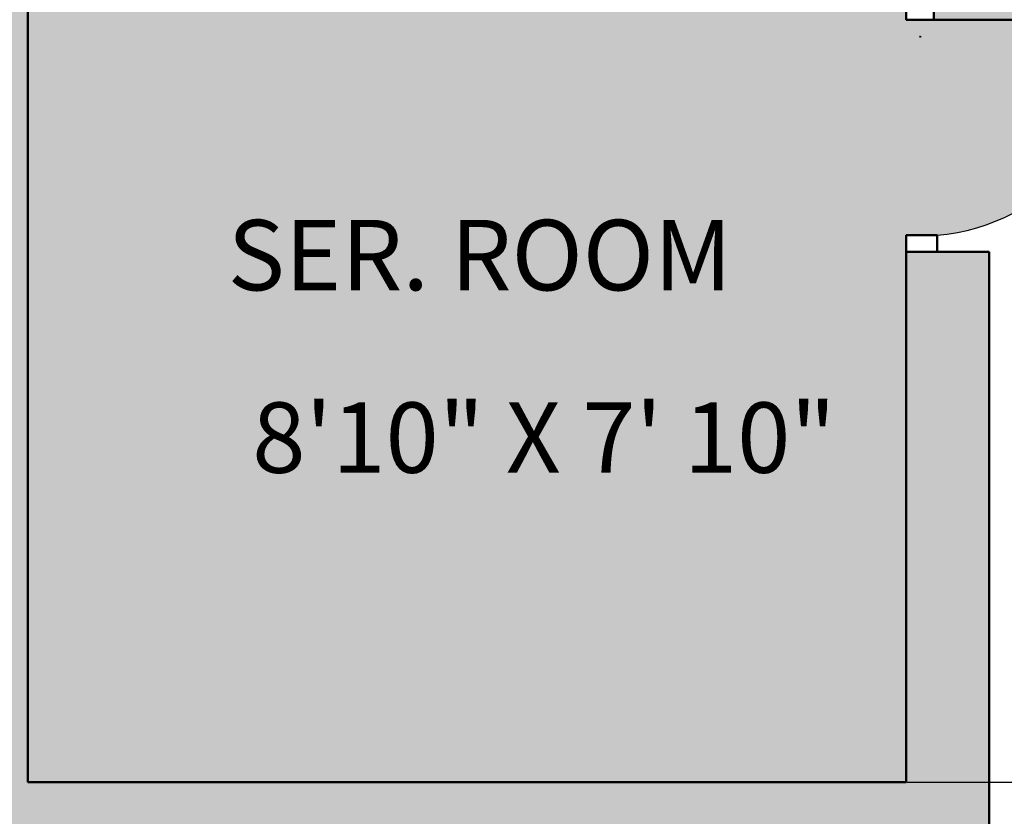
# Model space of a CAD drawing. Units: inches. Extents: x 925 to 2834, y 111 to 1355.
# Tile 9 of 25: x 1602 to 1721, y 723 to 820. Entities that reach past the tile are written whole.
import ezdxf

# ---------------------------------------------------------------- set-up
doc = ezdxf.new("R2010")
doc.units = ezdxf.units.IN
doc.header["$MEASUREMENT"] = 0
for name, color, linetype, lineweight in [('A-ANNO-DIMS', 2, 'Continuous', 18), ('A-AREA-IDEN', 7, 'Continuous', 18), ('A-DOOR', 2, 'Continuous', 25), ('A-FLOR-PATT', 252, 'Continuous', 13), ('A-WALL', 7, 'Continuous', 50)]:
    doc.layers.add(name, color=color, linetype=linetype, lineweight=lineweight)
doc.styles.get("Standard").update_dxf_attribs({"font": 'arial.ttf'})
doc.dimstyles.get("Standard").update_dxf_attribs({"dimtxt": 6, "dimasz": 3, "dimexe": 0.18, "dimexo": 0.0625, "dimgap": 0.09, "dimtad": 0, "dimtih": 1, "dimtoh": 1, "dimdec": 1, "dimzin": 0, "dimdsep": 46, "dimlunit": 3, "dimtxsty": 'Standard', "dimblk": 'ARCHTICK', "dimcen": 0.09, "dimadec": 0, "dimazin": 0, "dimtfac": 1, "dimtdec": 1, "dimtofl": 0, "dimtmove": 0, "dimatfit": 3, "dimfxl": 1, "dimtolj": 1, "dimtzin": 0, "dimarcsym": 0})

# ---------------------------------------------------------------- blocks, each defined once
blk = doc.blocks.new('_ArchTick')
at = {"color": 0, "linetype": 'ByBlock', "const_width": 0.15}
blk.add_lwpolyline([(-0.5, -0.5), (0.5, 0.5)], dxfattribs=at)
blk = doc.blocks.new('*D45')
at = {"layer": 'A-ANNO-DIMS', "color": 0, "lineweight": -2, "transparency": 16777216}
for p, q in [((1708.78, 727.59), (1988.62, 727.59)), ((1988.44, 727.59), (1988.44, 687.74)), ((1988.44, 641.59), (1988.44, 681.44)), ((1708.78, 641.59), (1988.62, 641.59))]:
    blk.add_line(p, q, dxfattribs=at)
at = {"layer": 'Defpoints', "color": 0, "transparency": 16777216}
for p in [(1708.71, 727.59), (1988.44, 727.59), (1708.71, 641.59)]:
    blk.add_point(p, dxfattribs=at)
at = {"layer": 'A-ANNO-DIMS', "color": 0, "lineweight": -2, "transparency": 16777216, "xscale": 3, "yscale": 3, "zscale": 3}
for p, rotation in [((1988.44, 727.59), 90), ((1988.44, 641.59), 270)]:
    blk.add_blockref('_ArchTick', p, dxfattribs=dict(at, rotation=rotation))
at = {"layer": 'A-ANNO-DIMS', "color": 0, "transparency": 16777216, "insert": (1988.44, 684.59), "char_height": 6, "attachment_point": 5}
blk.add_mtext('\\A1;86', dxfattribs=at)
blk = doc.blocks.new('*D46')
at = {"layer": 'A-ANNO-DIMS', "color": 0, "lineweight": -2, "transparency": 16777216}
for p, q in [((1708.78, 828.59), (1988.62, 828.59)), ((1988.44, 828.59), (1988.44, 781.24)), ((1988.44, 727.59), (1988.44, 774.94)), ((1708.78, 727.59), (1988.62, 727.59))]:
    blk.add_line(p, q, dxfattribs=at)
at = {"layer": 'Defpoints', "color": 0, "transparency": 16777216}
for p in [(1708.71, 828.59), (1988.44, 828.59), (1708.71, 727.59)]:
    blk.add_point(p, dxfattribs=at)
at = {"layer": 'A-ANNO-DIMS', "color": 0, "lineweight": -2, "transparency": 16777216, "xscale": 3, "yscale": 3, "zscale": 3}
for p, rotation in [((1988.44, 828.59), 90), ((1988.44, 727.59), 270)]:
    blk.add_blockref('_ArchTick', p, dxfattribs=dict(at, rotation=rotation))
at = {"layer": 'A-ANNO-DIMS', "color": 0, "transparency": 16777216, "insert": (1988.44, 778.09), "char_height": 6, "attachment_point": 5}
blk.add_mtext('\\A1;101', dxfattribs=at)
blk = doc.blocks.new('*D82')
at = {"layer": 'A-ANNO-DIMS', "color": 0, "lineweight": -2, "transparency": 16777216}
for p, q in [((1710.41, 817.46), (1710.41, 817.64)), ((1710.32, 817.55), (1710.5, 817.55)), ((1739.82, 792.74), (1728.79, 802.05)), ((1742.82, 792.74), (1739.82, 792.74))]:
    blk.add_line(p, q, dxfattribs=at)
at = {"layer": 'Defpoints', "color": 0, "transparency": 16777216}
for p in [(1710.41, 817.55), (1728.79, 802.05)]:
    blk.add_point(p, dxfattribs=at)
at = {"layer": 'A-ANNO-DIMS', "color": 0, "lineweight": -2, "transparency": 16777216, "xscale": 3, "yscale": 3, "zscale": 3, "rotation": 139.8500923460391}
blk.add_blockref('_ArchTick', (1728.79, 802.05), dxfattribs=at)
at = {"layer": 'A-ANNO-DIMS', "color": 0, "transparency": 16777216, "insert": (1762.43, 792.74), "char_height": 6, "attachment_point": 5}
blk.add_mtext('\\A1;2X R24.05', dxfattribs=at)

msp = doc.modelspace()

# ---------------------------------------------------------------- hatches: boundary and pattern name
at = {"layer": 'A-FLOR-PATT', "transparency": 33554605}
h = msp.add_hatch(color=256, dxfattribs=at)
h.dxf.hatch_style = 1
h.paths.add_polyline_path([(1931.688, 1294.5638), (991.7375, 1294.5638), (991.7375, 172.1134), (1931.688, 172.1134)])
h.paths.add_polyline_path([(1910.7128, 1273.5886), (1910.7128, 193.0886), (1012.7128, 193.0886), (1012.7128, 1273.5886)], flags=16)
h.paths.add_polyline_path([(1850.7128, 1213.5886), (1850.7128, 253.0886), (1072.7128, 253.0886), (1072.7128, 1213.5886)], flags=0)
h.paths.add_polyline_path([(1838.7128, 1201.5886), (1838.7128, 265.0886), (1084.7128, 265.0886), (1084.7128, 530.5886), (1084.7128, 1201.5886)], flags=0)
h.paths.add_polyline_path([(1547.6758, 1155.7396), (1547.6758, 1119.115), (1513.0687, 1119.115), (1513.0687, 1155.7396)], flags=0)
h.paths.add_polyline_path([(1600.1067, 1154.9439), (1634.7139, 1154.9439), (1634.7139, 1119.115), (1600.1067, 1119.115)], flags=0)
h.paths.add_polyline_path([(1505.2502, 1144.5358), (1505.2502, 1119.115), (1470.643, 1119.115), (1470.643, 1144.5358)], flags=0)
h.paths.add_polyline_path([(1559.1357, 1141.0962), (1593.7428, 1141.0962), (1593.7428, 1119.115), (1559.1357, 1119.115)], flags=0)
h.paths.add_polyline_path([(1462.8966, 1154.9439), (1462.8966, 1119.115), (1428.2895, 1119.115), (1428.2895, 1154.9439)], flags=0)
h.paths.add_polyline_path([(1642.4603, 1144.5358), (1677.0675, 1144.5358), (1677.0675, 1119.115), (1642.4603, 1119.115)], flags=0)
h.paths.add_polyline_path([(1422.3508, 1141.0962), (1422.3508, 1119.115), (1387.7436, 1119.115), (1387.7436, 1141.0962)], flags=0)
h.paths.add_polyline_path([(1684.8859, 1155.7396), (1719.4931, 1155.7396), (1719.4931, 1119.115), (1684.8859, 1119.115)], flags=0)
h.paths.add_polyline_path([(1718.7128, 1081.5886), (1718.7128, 1050.1249), (1715.7128, 1050.1249), (1715.7128, 1026.1249), (1715.7128, 1002.1249), (1718.7128, 1002.1249), (1730.7128, 1002.1249), (1730.7128, 998.1249), (1730.7128, 990.1249), (1730.7128, 986.1249), (1718.7128, 986.1249), (1718.7128, 893.5886), (1715.3735, 893.5886), (1715.3735, 891.5886), (1713.3735, 891.5886, 0.41421356), (1677.3735, 855.5886), (1713.3735, 855.5886), (1713.3735, 853.5886), (1715.3735, 853.5886), (1715.3735, 851.5886), (1718.7128, 851.5886), (1718.7128, 821.5865), (1734.4655, 821.5865), (1734.3735, 819.5886, -0.41421356), (1712.4415, 793.5886), (1712.4415, 791.5886), (1718.7128, 791.5886), (1718.7128, 717.5886), (1718.7128, 669.5886), (1732.7128, 669.5886), (1732.7128, 665.5886), (1732.7128, 641.5886), (1732.7128, 634.5886), (1732.7128, 610.5886), (1732.7128, 603.5886), (1718.7128, 603.5886), (1718.7128, 385.0886), (1434.2128, 385.0886), (1434.2128, 530.5886), (1410.2128, 530.5886), (1408.2128, 530.5886), (1408.2128, 532.5886, 0.41421356), (1372.2128, 568.5886), (1372.2128, 532.5886), (1370.2128, 532.5886), (1370.2128, 530.5886), (1368.2128, 530.5886), (1282.2128, 530.5886), (1210.2128, 530.5886), (1200.2128, 530.5886), (1200.2128, 542.1915), (1183.2307, 542.1915), (1183.2307, 546.1915), (1200.2128, 546.1915), (1200.2128, 572.1915), (1183.2307, 572.1915), (1183.2307, 576.1915), (1200.2128, 576.1915), (1200.2128, 727.5886), (1210.2128, 727.5886), (1234.2128, 727.5886), (1259.7128, 727.5886), (1259.7128, 775.5886), (1259.7128, 799.5886), (1259.7128, 847.5886), (1259.7128, 993.5872), (1259.7128, 1065.5872), (1259.7128, 1071.5886), (1219.6318, 1071.5886), (1219.6318, 1081.5886), (1084.7128, 1081.5886), (1084.7128, 1119.115), (1256.8974, 1119.115), (1256.8974, 1154.9439), (1291.5046, 1154.9439), (1291.5046, 1119.115), (1256.8974, 1119.115), (1256.6723, 1081.5886), (1293.7128, 1081.5886), (1341.7128, 1081.5886), (1341.7128, 1093.5886), (1347.7128, 1093.5886), (1371.7128, 1093.5886), (1377.7128, 1093.5886), (1377.7128, 1081.5886), (1668.7128, 1081.5886), (1668.7128, 1117.5886), (1675.7128, 1117.5886), (1711.7128, 1117.5886), (1718.7128, 1117.5886)], flags=0)
h.paths.add_polyline_path([(1376.2838, 1155.7396), (1376.2838, 1119.115), (1341.6766, 1119.115), (1341.6766, 1155.7396)], flags=0)
h.paths.add_polyline_path([(1341.7128, 1076.0886), (1293.7128, 1076.0886), (1293.7128, 1071.5886), (1269.7128, 1071.5886), (1269.7128, 1065.5872), (1266.7128, 1065.5872), (1266.7128, 1029.5872), (1265.7128, 1029.5872), (1265.7128, 993.5872), (1269.7128, 993.5872), (1269.7128, 903.5886), (1269.7128, 893.5886), (1269.7128, 847.5886), (1265.2128, 847.5886), (1265.2128, 799.5886), (1269.7128, 799.5886), (1269.7128, 775.5886), (1265.2128, 775.5886), (1265.2128, 727.5886), (1269.7128, 727.5886), (1444.2128, 727.5886), (1444.2128, 717.5886), (1234.2128, 717.5886), (1234.2128, 722.0886), (1210.2128, 722.0886), (1210.2128, 717.5886), (1210.2128, 540.5886), (1210.2128, 536.0886), (1282.2128, 536.0886), (1282.2128, 535.0886), (1210.2128, 535.0886), (1210.2128, 540.5886), (1210.2128, 717.5886), (1210.2128, 723.0886), (1234.2128, 723.0886), (1234.2128, 717.5886), (1444.2128, 717.5886), (1444.2128, 727.5886), (1269.7128, 727.5886), (1264.2128, 727.5886), (1264.2128, 775.5886), (1269.7128, 775.5886), (1269.7128, 799.5886), (1264.2128, 799.5886), (1264.2128, 847.5886), (1269.7128, 847.5886), (1269.7128, 893.5886), (1269.7128, 903.5886), (1269.7128, 993.5872), (1264.7128, 993.5872), (1264.7128, 1029.5872), (1265.7128, 1029.5872), (1265.7128, 1065.5872), (1269.7128, 1065.5872), (1269.7128, 1071.5886), (1293.7128, 1071.5886), (1293.7128, 1077.0886), (1341.7128, 1077.0886)], flags=0)
h.paths.add_polyline_path([(1730.9529, 1141.0962), (1765.5601, 1141.0962), (1765.5601, 1119.115), (1730.9529, 1119.115)], flags=0)
h.paths.add_polyline_path([(1333.8582, 1144.5358), (1333.8582, 1119.115), (1299.251, 1119.115), (1299.251, 1144.5358)], flags=0)
h.paths.add_polyline_path([(1592.7128, 968.5886), (1596.0342, 968.5886), (1602.7128, 968.5886), (1708.7128, 968.5886), (1708.7128, 903.5886), (1602.7128, 903.5886), (1602.7128, 938.5886), (1592.7128, 938.5886), (1592.7128, 903.5886), (1451.7128, 903.5886), (1451.7128, 893.5886), (1511.7128, 893.5886), (1511.7128, 881.5886), (1515.2128, 881.5886), (1518.7128, 881.5886), (1518.7128, 893.5886), (1592.7128, 893.5886), (1592.7128, 799.5886), (1518.7128, 799.5886), (1518.7128, 857.5886), (1511.7128, 857.5886), (1511.7128, 799.5886), (1511.7128, 772.0886), (1521.7128, 772.0886), (1521.7128, 792.5886), (1592.7128, 792.5886), (1592.7128, 727.5886), (1521.7128, 727.5886), (1521.7128, 748.0886), (1511.7128, 748.0886), (1511.7128, 717.5886), (1708.7128, 717.5886), (1714.2128, 717.5886), (1714.2128, 669.5886), (1708.7128, 669.5886), (1708.7128, 641.5886), (1492.2128, 641.5886), (1492.2128, 631.5886), (1621.2128, 631.5886), (1621.2128, 443.0886), (1625.7128, 443.0886), (1625.7128, 503.0886), (1625.7128, 507.5886), (1625.7128, 631.5886), (1708.7128, 631.5886), (1708.7128, 507.5886), (1655.7128, 507.5886), (1655.7128, 503.0886), (1708.7128, 503.0886), (1708.7128, 395.0886), (1625.7128, 395.0886), (1625.7128, 419.0886), (1621.2128, 419.0886), (1621.2128, 395.0886), (1482.2128, 395.0886), (1482.2128, 385.0886), (1434.2128, 385.0886), (1434.2128, 433.0886), (1444.2128, 433.0886), (1444.2128, 631.5886), (1450.2128, 631.5886), (1450.2128, 634.91), (1452.2128, 634.91), (1452.2128, 669.5886), (1454.2128, 669.5886, -0.40021217), (1490.1712, 635.3173), (1492.2128, 635.3173), (1492.2128, 641.5886), (1564.7128, 641.5886), (1564.7128, 677.5886), (1672.7128, 677.5886), (1672.7128, 681.5886), (1564.7128, 681.5886), (1564.7128, 717.5886), (1511.7128, 717.5886), (1511.7128, 748.0886), (1511.7128, 772.0886), (1511.7128, 799.5886), (1511.7128, 857.5886), (1511.8913, 857.5886), (1511.8913, 859.5886), (1515.6201, 859.5886, 0.41421356), (1537.552, 879.5886), (1513.552, 879.5886), (1511.8913, 879.5886), (1511.8913, 881.5886), (1511.7128, 881.5886), (1511.7128, 893.5886), (1451.7128, 893.5886), (1451.7128, 903.5886), (1592.7128, 903.5886), (1592.7128, 938.5886), (1592.7128, 940.5886), (1596.4415, 940.5886, 0.41421356), (1618.3735, 966.5886), (1594.3735, 966.5886), (1592.7128, 966.5886)], flags=0)
h.paths.add_polyline_path([(1377.7128, 903.5886), (1377.7128, 893.5886), (1305.7128, 893.5886), (1305.7128, 903.5886)], flags=0)
h.paths.add_polyline_path([(1708.7128, 821.5886), (1712.0342, 821.5886), (1712.0342, 819.5886), (1710.3735, 819.5886), (1708.7128, 819.5886)], flags=0)
h.paths.add_polyline_path([(1576.7128, 695.1992), (1575.5896, 693.6649), (1575.9687, 694.6994), (1575.4438, 695.1992), (1575.9687, 695.699), (1575.5896, 696.7335)], flags=0)
h.paths.add_polyline_path([(1565.9817, 662.3134), (1565.4568, 661.8136), (1565.8359, 660.7791), (1564.7128, 662.3134), (1565.8359, 663.8477), (1565.4568, 662.8132)], flags=0)
h.paths.add_polyline_path([(1444.2128, 433.0886), (1444.2128, 395.0886), (1482.2128, 395.0886), (1482.2128, 389.0886), (1438.2128, 389.0886), (1438.2128, 391.8608), (1438.2128, 433.0886)], flags=0)
h.paths.add_polyline_path([(1410.2128, 506.5886), (1410.2128, 289.0886), (1108.7128, 289.0886), (1108.7128, 506.5886)], flags=0)
h.paths.add_polyline_path([(1612.3153, 838.3016), (1680.4151, 838.3016), (1680.4151, 851.3131), (1612.3153, 851.3131)], flags=8)
h.paths.add_polyline_path([(1208.3174, 395.0436), (1282.1017, 395.0436), (1282.1017, 408.0552), (1208.3174, 408.0552)], flags=8)
h.paths.add_polyline_path([(1291.8049, 598.7427), (1369.8017, 598.7427), (1369.8017, 611.7542), (1291.8049, 611.7542)], flags=8)
h.paths.add_polyline_path([(1119.679, 917.3022), (1191.0817, 917.3022), (1191.0817, 930.3137), (1119.679, 930.3137)], flags=8)
h.paths.add_polyline_path([(1332.2261, 815.9808), (1410.2258, 815.9808), (1410.2258, 829.001), (1332.2261, 829.001)], flags=8)
h.paths.add_polyline_path([(1390.9013, 955.8158), (1475.4981, 955.8158), (1475.4981, 968.8273), (1390.9013, 968.8273)], flags=8)
h.paths.add_polyline_path([(1620.3436, 998.9325), (1688.4434, 998.9325), (1688.4434, 1011.944), (1620.3436, 1011.944)], flags=8)
h.paths.add_polyline_path([(1620.3436, 914.1039), (1691.7405, 914.1039), (1691.7405, 927.1155), (1620.3436, 927.1155)], flags=8)
h.paths.add_polyline_path([(1521.4542, 816.005), (1589.5569, 816.005), (1589.5569, 829.0253), (1521.4542, 829.0253)], flags=8)
h.paths.add_polyline_path([(1528.524, 740.3497), (1602.3082, 740.3497), (1602.3082, 753.3613), (1528.524, 753.3613)], flags=8)
h.paths.add_polyline_path([(1627.6094, 762.6128), (1702.3091, 762.6128), (1702.3091, 775.6244), (1627.6094, 775.6244)], flags=8)
h.paths.add_polyline_path([(1610.5442, 657.2751), (1684.3284, 657.2751), (1684.3284, 670.2867), (1610.5442, 670.2867)], flags=8)
h.paths.add_polyline_path([(1636.6983, 519.472), (1711.3981, 519.472), (1711.3981, 532.4835), (1636.6983, 532.4835)], flags=8)
h.paths.add_polyline_path([(1616.8577, 424.8539), (1694.8545, 424.8539), (1694.8545, 437.8654), (1616.8577, 437.8654)], flags=8)
h.paths.add_polyline_path([(1506.1456, 460.8838), (1579.9299, 460.8838), (1579.9299, 473.8953), (1506.1456, 473.8953)], flags=8)
h.paths.add_polyline_path([(1624.6119, 784.6011), (1696.9185, 784.6011), (1696.9185, 797.7864), (1624.6119, 797.7864)], flags=8)
h.paths.add_polyline_path([(1606.3732, 854.2194), (1683.3039, 854.2194), (1683.3039, 867.4048), (1606.3732, 867.4048)], flags=8)
h.paths.add_polyline_path([(1127.8008, 940.3581), (1165.1637, 940.3581), (1165.1637, 953.5348), (1127.8008, 953.5348)], flags=8)
h.paths.add_polyline_path([(1620.8657, 1019.4968), (1677.3447, 1019.4968), (1677.3447, 1032.6735), (1620.8657, 1032.6735)], flags=8)
h.paths.add_polyline_path([(1620.8643, 930.1821), (1703.0564, 930.1821), (1703.0564, 943.3675), (1620.8643, 943.3675)], flags=8)
h.paths.add_polyline_path([(1324.5702, 836.8338), (1408.0892, 836.8338), (1408.0892, 850.0191), (1324.5702, 850.0191)], flags=8)
h.paths.add_polyline_path([(1281.6584, 622.8885), (1383.6213, 622.8885), (1383.6213, 636.0739), (1281.6584, 636.0739)], flags=8)
h.paths.add_polyline_path([(1210.6721, 416.7893), (1269.1299, 416.7893), (1269.1299, 429.9747), (1210.6721, 429.9747)], flags=8)
h.paths.add_polyline_path([(1507.8264, 477.4836), (1586.7329, 477.4836), (1586.7329, 490.669), (1507.8264, 490.669)], flags=8)
h.paths.add_polyline_path([(1643.6238, 443.8135), (1696.6696, 443.8135), (1696.6696, 456.5643), (1643.6238, 456.5643)], flags=8)
h.paths.add_polyline_path([(1647.2466, 540.5638), (1693.1825, 540.5638), (1693.1825, 553.7491), (1647.2466, 553.7491)], flags=8)
h.paths.add_polyline_path([(1626.0633, 668.5064), (1673.3174, 668.5064), (1673.3174, 681.6831), (1626.0633, 681.6831)], flags=8)
h.paths.add_polyline_path([(1538.2915, 830.7872), (1567.5942, 830.7872), (1567.5942, 843.5293), (1538.2915, 843.5293)], flags=8)
h.paths.add_polyline_path([(1530.9338, 754.0477), (1559.576, 754.0477), (1559.576, 766.7898), (1530.9338, 766.7898)], flags=8)
h.paths.add_polyline_path([(1351.2461, 979.2309), (1513.8919, 979.2309), (1513.8919, 992.4076), (1351.2461, 992.4076)], flags=8)
at = {"layer": 'A-FLOR-PATT'}
h = msp.add_hatch(color=256, dxfattribs=at)
h.dxf.hatch_style = 1
h.paths.add_polyline_path([(1850.7128, 1213.5886), (1072.7128, 1213.5886), (1072.7128, 253.0886), (1850.7128, 253.0886)])
h.paths.add_polyline_path([(1084.7128, 1201.5886), (1838.7128, 1201.5886), (1838.7128, 265.0886), (1084.7128, 265.0886)], flags=16)
h.paths.add_polyline_path([(1183.2307, 576.1915), (1200.2128, 576.1915), (1200.2128, 727.5886), (1210.2128, 727.5886), (1234.2128, 727.5886), (1259.7128, 727.5886), (1259.7128, 775.5886), (1259.7128, 799.5886), (1259.7128, 847.5886), (1259.7128, 993.5872), (1259.7128, 1065.5872), (1259.7128, 1071.5886), (1219.6318, 1071.5886), (1219.6318, 1081.5886), (1293.7128, 1081.5886), (1341.7128, 1081.5886), (1341.7128, 1093.5886), (1347.7128, 1093.5886), (1347.7128, 1081.5886), (1371.7128, 1081.5886), (1371.7128, 1093.5886), (1377.7128, 1093.5886), (1377.7128, 1081.5886), (1668.7128, 1081.5886), (1668.7128, 1117.5886), (1675.7128, 1117.5886), (1675.7128, 1081.5886), (1711.7128, 1081.5886), (1711.7128, 1117.5886), (1718.7128, 1117.5886), (1718.7128, 1081.5886), (1718.7128, 1050.1249), (1715.7128, 1050.1249), (1715.7128, 1026.1249), (1715.7128, 1002.1249), (1718.7128, 1002.1249), (1730.7128, 1002.1249), (1730.7128, 998.1249), (1730.7128, 990.1249), (1730.7128, 986.1249), (1718.7128, 986.1249), (1718.7128, 893.5886), (1715.3735, 893.5886), (1715.3735, 891.5886), (1713.3735, 891.5886, 0.41421356), (1677.3735, 855.5886), (1713.3735, 855.5886), (1713.3735, 853.5886), (1715.3735, 853.5886), (1715.3735, 851.5886), (1718.7128, 851.5886), (1718.7128, 821.5865), (1734.4655, 821.5865), (1734.3735, 819.5886, -0.41421356), (1712.4415, 793.5886), (1712.4415, 791.5886), (1718.7128, 791.5886), (1718.7128, 717.5886), (1718.7128, 669.5886), (1732.7128, 669.5886), (1732.7128, 665.5886), (1732.7128, 641.5886), (1732.7128, 634.5886), (1732.7128, 610.5886), (1732.7128, 603.5886), (1718.7128, 603.5886), (1718.7128, 385.0886), (1434.2128, 385.0886), (1434.2128, 433.0886), (1434.2128, 530.5886), (1410.2128, 530.5886), (1408.2128, 530.5886), (1408.2128, 532.5886, 0.41421356), (1372.2128, 568.5886), (1372.2128, 532.5886), (1370.2128, 532.5886), (1370.2128, 530.5886), (1368.2128, 530.5886), (1282.2128, 530.5886), (1210.2128, 530.5886), (1200.2128, 530.5886), (1200.2128, 542.1915), (1183.2307, 542.1915), (1183.2307, 546.1915), (1200.2128, 546.1915), (1200.2128, 572.1915), (1183.2307, 572.1915)], flags=0)
h.paths.add_polyline_path([(1210.2128, 717.5886), (1210.2128, 723.0886), (1234.2128, 723.0886), (1234.2128, 717.5886), (1444.2128, 717.5886), (1444.2128, 727.5886), (1269.7128, 727.5886), (1264.2128, 727.5886), (1264.2128, 775.5886), (1269.7128, 775.5886), (1269.7128, 799.5886), (1264.2128, 799.5886), (1264.2128, 847.5886), (1269.7128, 847.5886), (1269.7128, 893.5886), (1269.7128, 903.5886), (1269.7128, 993.5872), (1264.7128, 993.5872), (1264.7128, 1029.5872), (1265.7128, 1029.5872), (1265.7128, 1065.5872), (1269.7128, 1065.5872), (1269.7128, 1071.5886), (1293.7128, 1071.5886), (1293.7128, 1077.0886), (1341.7128, 1077.0886), (1341.7128, 1076.0886), (1293.7128, 1076.0886), (1293.7128, 1071.5886), (1269.7128, 1071.5886), (1269.7128, 1065.5872), (1266.7128, 1065.5872), (1266.7128, 1029.5872), (1265.7128, 1029.5872), (1265.7128, 993.5872), (1269.7128, 993.5872), (1269.7128, 903.5886), (1269.7128, 893.5886), (1269.7128, 847.5886), (1265.2128, 847.5886), (1265.2128, 799.5886), (1269.7128, 799.5886), (1269.7128, 775.5886), (1265.2128, 775.5886), (1265.2128, 727.5886), (1269.7128, 727.5886), (1444.2128, 727.5886), (1444.2128, 717.5886), (1234.2128, 717.5886), (1234.2128, 722.0886), (1210.2128, 722.0886), (1210.2128, 717.5886), (1210.2128, 540.5886), (1210.2128, 536.0886), (1282.2128, 536.0886), (1282.2128, 535.0886), (1210.2128, 535.0886), (1210.2128, 540.5886)], flags=0)
h.paths.add_polyline_path([(1450.2128, 634.91), (1452.2128, 634.91), (1452.2128, 669.5886), (1454.2128, 669.5886, -0.40021217), (1490.1712, 635.3173), (1492.2128, 635.3173), (1492.2128, 641.5886), (1564.7128, 641.5886), (1564.7128, 677.5886), (1672.7128, 677.5886), (1672.7128, 681.5886), (1564.7128, 681.5886), (1564.7128, 717.5886), (1511.7128, 717.5886), (1511.7128, 748.0886), (1511.7128, 772.0886), (1511.7128, 799.5886), (1511.7128, 857.5886), (1511.8913, 857.5886), (1511.8913, 859.5886), (1515.6201, 859.5886, 0.41421356), (1537.552, 879.5886), (1513.552, 879.5886), (1511.8913, 879.5886), (1511.8913, 881.5886), (1511.7128, 881.5886), (1511.7128, 893.5886), (1451.7128, 893.5886), (1451.7128, 903.5886), (1592.7128, 903.5886), (1592.7128, 938.5886), (1592.7128, 940.5886), (1596.4415, 940.5886, 0.41421356), (1618.3735, 966.5886), (1594.3735, 966.5886), (1592.7128, 966.5886), (1592.7128, 968.5886), (1596.0342, 968.5886), (1602.7128, 968.5886), (1708.7128, 968.5886), (1708.7128, 903.5886), (1602.7128, 903.5886), (1602.7128, 938.5886), (1592.7128, 938.5886), (1592.7128, 903.5886), (1451.7128, 903.5886), (1451.7128, 893.5886), (1511.7128, 893.5886), (1511.7128, 881.5886), (1518.7128, 881.5886), (1518.7128, 893.5886), (1592.7128, 893.5886), (1592.7128, 799.5886), (1518.7128, 799.5886), (1518.7128, 857.5886), (1511.7128, 857.5886), (1511.7128, 799.5886), (1511.7128, 772.0886), (1521.7128, 772.0886), (1521.7128, 792.5886), (1592.7128, 792.5886), (1592.7128, 727.5886), (1521.7128, 727.5886), (1521.7128, 748.0886), (1511.7128, 748.0886), (1511.7128, 717.5886), (1708.7128, 717.5886), (1714.2128, 717.5886), (1714.2128, 669.5886), (1708.7128, 669.5886), (1708.7128, 641.5886), (1492.2128, 641.5886), (1492.2128, 631.5886), (1621.2128, 631.5886), (1621.2128, 443.0886), (1625.7128, 443.0886), (1625.7128, 503.0886), (1625.7128, 507.5886), (1625.7128, 631.5886), (1708.7128, 631.5886), (1708.7128, 507.5886), (1655.7128, 507.5886), (1655.7128, 503.0886), (1708.7128, 503.0886), (1708.7128, 395.0886), (1625.7128, 395.0886), (1625.7128, 419.0886), (1621.2128, 419.0886), (1621.2128, 395.0886), (1482.2128, 395.0886), (1482.2128, 389.0886), (1438.2128, 389.0886), (1438.2128, 391.8608), (1438.2128, 433.0886), (1444.2128, 433.0886), (1444.2128, 631.5886), (1450.2128, 631.5886)], flags=0)
h.paths.add_polyline_path([(1444.2128, 433.0886), (1444.2128, 395.0886), (1482.2128, 395.0886), (1482.2128, 391.0886), (1440.2128, 391.0886), (1440.2128, 391.8608), (1440.2128, 433.0886)], flags=0)
h.paths.add_polyline_path([(1305.7128, 893.5886), (1305.7128, 903.5886), (1377.7128, 903.5886), (1377.7128, 893.5886)], flags=0)
h.paths.add_polyline_path([(1564.7128, 662.3134), (1565.8359, 663.8477), (1565.4568, 662.8132), (1565.9817, 662.3134), (1565.4568, 661.8136), (1565.8359, 660.7791)], flags=0)
h.paths.add_polyline_path([(1575.4438, 695.1992), (1575.9687, 695.699), (1575.5896, 696.7335), (1576.7128, 695.1992), (1575.5896, 693.6649), (1575.9687, 694.6994)], flags=0)
h.paths.add_polyline_path([(1708.7128, 821.5886), (1712.0342, 821.5886), (1712.0342, 819.5886), (1710.3735, 819.5886), (1708.7128, 819.5886)], flags=0)
h = msp.add_hatch(color=256, dxfattribs=at)
h.dxf.hatch_style = 1
h.paths.add_polyline_path([(1718.7128, 603.5886), (1708.7128, 603.5886), (1708.7128, 507.5886), (1655.7128, 507.5886), (1655.7128, 503.0886), (1708.7128, 503.0886), (1708.7128, 395.0886), (1625.7128, 395.0886), (1625.7128, 419.0886), (1621.2128, 419.0886), (1621.2128, 395.0886), (1482.2128, 395.0886), (1482.2128, 385.0886), (1718.7128, 385.0886)])
h.paths.add_polyline_path([(1625.7128, 631.5886), (1708.7128, 631.5886), (1708.7128, 603.5886), (1718.7128, 603.5886), (1732.7128, 603.5886), (1732.7128, 610.5886), (1715.7128, 610.5886), (1715.7128, 634.5886), (1732.7128, 634.5886), (1732.7128, 641.5886), (1715.7128, 641.5886), (1715.7128, 665.5886), (1732.7128, 665.5886), (1732.7128, 669.5886), (1708.7128, 669.5886), (1708.7128, 641.5886), (1492.2128, 641.5886), (1492.2128, 631.5886), (1621.2128, 631.5886), (1621.2128, 443.0886), (1625.7128, 443.0886), (1625.7128, 503.0886), (1625.7128, 507.5886)])
h.paths.add_polyline_path([(1718.7128, 851.5886), (1708.7128, 851.5886), (1708.7128, 828.5886), (1602.7128, 828.5886), (1602.7128, 893.5886), (1708.7128, 893.5886), (1718.7128, 893.5886), (1718.7128, 986.1249), (1730.7128, 986.1249), (1730.7128, 990.1249), (1718.7128, 990.1249), (1718.7128, 998.1249), (1730.7128, 998.1249), (1730.7128, 1002.1249), (1718.7128, 1002.1249), (1708.7128, 1002.1249), (1708.7128, 975.5886), (1602.7128, 975.5886), (1602.7128, 1011.5886), (1592.7128, 1011.5886), (1592.7128, 968.5886), (1596.0342, 968.5886), (1602.7128, 968.5886), (1708.7128, 968.5886), (1708.7128, 903.5886), (1602.7128, 903.5886), (1602.7128, 938.5886), (1592.7128, 938.5886), (1592.7128, 903.5886), (1451.7128, 903.5886), (1451.7128, 893.5886), (1511.7128, 893.5886), (1511.7128, 881.5886), (1515.2128, 881.5886), (1518.7128, 881.5886), (1518.7128, 893.5886), (1592.7128, 893.5886), (1592.7128, 799.5886), (1518.7128, 799.5886), (1518.7128, 857.5886), (1511.7128, 857.5886), (1511.7128, 799.5886), (1511.7128, 772.0886), (1521.7128, 772.0886), (1521.7128, 792.5886), (1592.7128, 792.5886), (1592.7128, 727.5886), (1521.7128, 727.5886), (1521.7128, 748.0886), (1511.7128, 748.0886), (1511.7128, 717.5886), (1708.7128, 717.5886), (1718.7128, 717.5886), (1718.7128, 727.5886), (1718.7128, 791.5886), (1708.7128, 791.5886), (1708.7128, 727.5886), (1602.7128, 727.5886), (1602.7128, 821.5886), (1708.7128, 821.5886), (1712.0342, 821.5886), (1718.7128, 821.5886)])
h.paths.add_polyline_path([(1718.7128, 1081.5886), (1718.7128, 1117.5886), (1711.7128, 1117.5886), (1711.7128, 1081.5886), (1675.7128, 1081.5886), (1675.7128, 1117.5886), (1668.7128, 1117.5886), (1668.7128, 1081.5886), (1377.7128, 1081.5886), (1377.7128, 1093.5886), (1371.7128, 1093.5886), (1371.7128, 1081.5886), (1347.7128, 1081.5886), (1347.7128, 1093.5886), (1341.7128, 1093.5886), (1341.7128, 1081.5886), (1341.7128, 1071.5886), (1592.7128, 1071.5886), (1592.7128, 1035.5886), (1602.7128, 1035.5886), (1602.7128, 1071.5886), (1708.7128, 1071.5886), (1708.7128, 1050.1249), (1718.7128, 1050.1249)])
h.paths.add_polyline_path([(1293.7128, 1081.5886), (1219.6318, 1081.5886), (1219.6318, 1071.5886), (1259.7128, 1071.5886), (1259.7128, 1065.5872), (1269.7128, 1065.5872), (1269.7128, 1071.5886), (1293.7128, 1071.5886)])
h.paths.add_polyline_path([(1269.7128, 903.5886), (1269.7128, 993.5872), (1259.7128, 993.5872), (1259.7128, 847.5886), (1269.7128, 847.5886), (1269.7128, 893.5886)])
h.paths.add_polyline_path([(1377.7128, 903.5886), (1305.7128, 903.5886), (1305.7128, 893.5886), (1377.7128, 893.5886)])
h.paths.add_polyline_path([(1444.2128, 727.5886), (1269.7128, 727.5886), (1259.7128, 727.5886), (1234.2128, 727.5886), (1234.2128, 717.5886), (1444.2128, 717.5886)])
h.paths.add_polyline_path([(1269.7128, 799.5886), (1259.7128, 799.5886), (1259.7128, 775.5886), (1269.7128, 775.5886)])
h.paths.add_polyline_path([(1444.2128, 631.5886), (1450.2128, 631.5886), (1450.2128, 634.91), (1450.2128, 641.5886), (1434.2128, 641.5886), (1434.2128, 540.5886), (1410.2128, 540.5886), (1410.2128, 530.5886), (1434.2128, 530.5886), (1434.2128, 433.0886), (1444.2128, 433.0886)])
h.paths.add_polyline_path([(1368.2128, 533.91), (1368.2128, 540.5886), (1282.2128, 540.5886), (1282.2128, 530.5886), (1368.2128, 530.5886)])
h.paths.add_polyline_path([(1210.2128, 717.5886), (1210.2128, 727.5886), (1200.2128, 727.5886), (1200.2128, 576.1915), (1183.2307, 576.1915), (1183.2307, 572.1915), (1200.2128, 572.1915), (1200.2128, 546.1915), (1183.2307, 546.1915), (1183.2307, 542.1915), (1200.2128, 542.1915), (1200.2128, 530.5886), (1210.2128, 530.5886), (1210.2128, 540.5886)])
at = {"layer": 'A-FLOR-PATT', "transparency": 33554605}
h = msp.add_hatch(color=256, dxfattribs=at)
h.dxf.hatch_style = 1
h.paths.add_polyline_path([(1621.2128, 631.5886), (1492.2128, 631.5886), (1490.2128, 631.5886), (1490.2128, 633.5886, 0.41421356), (1454.2128, 669.5886), (1454.2128, 633.5886), (1452.2128, 633.5886), (1452.2128, 631.5886), (1450.2128, 631.5886), (1444.2128, 631.5886), (1444.2128, 395.0886), (1482.2128, 395.0886), (1621.2128, 395.0886), (1621.2128, 419.0886), (1625.7128, 419.0886), (1625.7128, 395.0886), (1708.7128, 395.0886), (1708.7128, 503.0886), (1655.7128, 503.0886), (1655.7128, 507.5886), (1708.7128, 507.5886), (1708.7128, 631.5886), (1625.7128, 631.5886), (1625.7128, 507.5886), (1625.7128, 503.0886), (1625.7128, 443.0886), (1621.2128, 443.0886)])
h.paths.add_polyline_path([(1636.6983, 519.472), (1711.3981, 519.472), (1711.3981, 532.4835), (1636.6983, 532.4835)], flags=9)
h.paths.add_polyline_path([(1616.8577, 424.8539), (1694.8545, 424.8539), (1694.8545, 437.8654), (1616.8577, 437.8654)], flags=24)
h.paths.add_polyline_path([(1506.1456, 460.8838), (1579.9299, 460.8838), (1579.9299, 473.8953), (1506.1456, 473.8953)], flags=24)
h.paths.add_polyline_path([(1507.8264, 477.4836), (1586.7329, 477.4836), (1586.7329, 490.669), (1507.8264, 490.669)], flags=24)
h.paths.add_polyline_path([(1643.6238, 443.8135), (1696.6696, 443.8135), (1696.6696, 456.5643), (1643.6238, 456.5643)], flags=24)
h.paths.add_polyline_path([(1647.2466, 540.5638), (1693.1825, 540.5638), (1693.1825, 553.7491), (1647.2466, 553.7491)], flags=24)
h.paths.add_polyline_path([(1612.3153, 838.3016), (1680.4151, 838.3016), (1680.4151, 851.3131), (1612.3153, 851.3131)], flags=9)
h.paths.add_polyline_path([(1291.8049, 598.7427), (1369.8017, 598.7427), (1369.8017, 611.7542), (1291.8049, 611.7542)], flags=9)
h.paths.add_polyline_path([(1119.679, 917.3022), (1191.0817, 917.3022), (1191.0817, 930.3137), (1119.679, 930.3137)], flags=9)
h.paths.add_polyline_path([(1332.2261, 815.9808), (1410.2258, 815.9808), (1410.2258, 829.001), (1332.2261, 829.001)], flags=9)
h.paths.add_polyline_path([(1390.9013, 955.8158), (1475.4981, 955.8158), (1475.4981, 968.8273), (1390.9013, 968.8273)], flags=9)
h.paths.add_polyline_path([(1620.3436, 998.9325), (1688.4434, 998.9325), (1688.4434, 1011.944), (1620.3436, 1011.944)], flags=9)
h.paths.add_polyline_path([(1620.3436, 914.1039), (1691.7405, 914.1039), (1691.7405, 927.1155), (1620.3436, 927.1155)], flags=9)
h.paths.add_polyline_path([(1521.4542, 816.005), (1589.5569, 816.005), (1589.5569, 829.0253), (1521.4542, 829.0253)], flags=9)
h.paths.add_polyline_path([(1528.524, 740.3497), (1602.3082, 740.3497), (1602.3082, 753.3613), (1528.524, 753.3613)], flags=9)
h.paths.add_polyline_path([(1627.6094, 762.6128), (1702.3091, 762.6128), (1702.3091, 775.6244), (1627.6094, 775.6244)], flags=9)
h.paths.add_polyline_path([(1624.6119, 784.6011), (1696.9185, 784.6011), (1696.9185, 797.7864), (1624.6119, 797.7864)], flags=9)
h.paths.add_polyline_path([(1606.3732, 854.2194), (1683.3039, 854.2194), (1683.3039, 867.4048), (1606.3732, 867.4048)], flags=9)
h.paths.add_polyline_path([(1127.8008, 940.3581), (1165.1637, 940.3581), (1165.1637, 953.5348), (1127.8008, 953.5348)], flags=9)
h.paths.add_polyline_path([(1620.8657, 1019.4968), (1677.3447, 1019.4968), (1677.3447, 1032.6735), (1620.8657, 1032.6735)], flags=9)
h.paths.add_polyline_path([(1620.8643, 930.1821), (1703.0564, 930.1821), (1703.0564, 943.3675), (1620.8643, 943.3675)], flags=9)
h.paths.add_polyline_path([(1324.5702, 836.8338), (1408.0892, 836.8338), (1408.0892, 850.0191), (1324.5702, 850.0191)], flags=9)
h.paths.add_polyline_path([(1281.6584, 622.8885), (1383.6213, 622.8885), (1383.6213, 636.0739), (1281.6584, 636.0739)], flags=9)
h.paths.add_polyline_path([(1626.0633, 668.5064), (1673.3174, 668.5064), (1673.3174, 681.6831), (1626.0633, 681.6831)], flags=9)
h.paths.add_polyline_path([(1538.2915, 830.7872), (1567.5942, 830.7872), (1567.5942, 843.5293), (1538.2915, 843.5293)], flags=9)
h.paths.add_polyline_path([(1530.9338, 754.0477), (1559.576, 754.0477), (1559.576, 766.7898), (1530.9338, 766.7898)], flags=9)
h.paths.add_polyline_path([(1351.2461, 979.2309), (1513.8919, 979.2309), (1513.8919, 992.4076), (1351.2461, 992.4076)], flags=9)
h = msp.add_hatch(color=256, dxfattribs=at)
h.dxf.hatch_style = 1
h.paths.add_polyline_path([(1708.7128, 791.5886), (1708.7128, 793.5886), (1712.4415, 793.5886, 0.41421356), (1734.3735, 819.5886), (1710.3735, 819.5886), (1708.7128, 819.5886), (1708.7128, 821.5886), (1602.7128, 821.5886), (1602.7128, 727.5886), (1708.7128, 727.5886)])
h.paths.add_polyline_path([(1708.7128, 851.5886), (1712.052, 851.5886), (1712.052, 853.5886), (1677.3735, 853.5886), (1677.3735, 855.5886, -0.40021217), (1711.6447, 891.5471), (1711.6447, 893.5886), (1708.7128, 893.5886), (1602.7128, 893.5886), (1602.7128, 828.5886), (1708.7128, 828.5886)])
h.paths.add_polyline_path([(1708.7128, 968.5886), (1618.4656, 968.5886), (1618.3735, 966.5886, -0.41421356), (1596.4415, 940.5886), (1596.4415, 938.5886), (1602.7128, 938.5886), (1602.7128, 903.5886), (1708.7128, 903.5886)])
h.paths.add_polyline_path([(1708.7128, 717.5886), (1672.7128, 717.5886), (1672.7128, 641.5886), (1708.7128, 641.5886)])
h.paths.add_polyline_path([(1588.7128, 717.5886), (1576.7128, 717.5886), (1576.7128, 681.5886), (1588.7128, 681.5886)])
h.paths.add_polyline_path([(1576.7128, 717.5886), (1564.7128, 717.5886), (1564.7128, 695.1992), (1575.4438, 695.1992), (1575.9687, 695.699), (1575.5896, 696.7335), (1576.7128, 695.1992)])
h.paths.add_polyline_path([(1576.7128, 695.1992), (1575.5896, 693.6649), (1575.9687, 694.6994), (1575.4438, 695.1992), (1564.7128, 695.1992), (1564.7128, 681.5886), (1576.7128, 681.5886)])
h.paths.add_polyline_path([(1600.7128, 717.5886), (1588.7128, 717.5886), (1588.7128, 681.5886), (1600.7128, 681.5886)])
h.paths.add_polyline_path([(1612.7128, 717.5886), (1600.7128, 717.5886), (1600.7128, 681.5886), (1612.7128, 681.5886)])
h.paths.add_polyline_path([(1624.7128, 717.5886), (1612.7128, 717.5886), (1612.7128, 681.5886), (1624.7128, 681.5886)])
h.paths.add_polyline_path([(1636.7128, 717.5886), (1624.7128, 717.5886), (1624.7128, 681.5886), (1636.7128, 681.5886)])
h.paths.add_polyline_path([(1648.7128, 717.5886), (1636.7128, 717.5886), (1636.7128, 681.5886), (1648.7128, 681.5886)])
h.paths.add_polyline_path([(1660.7128, 717.5886), (1648.7128, 717.5886), (1648.7128, 681.5886), (1660.7128, 681.5886)])
h.paths.add_polyline_path([(1672.7128, 717.5886), (1660.7128, 717.5886), (1660.7128, 681.5886), (1672.7128, 681.5886)])
h.paths.add_polyline_path([(1576.7128, 662.3134), (1565.9817, 662.3134), (1565.4568, 661.8136), (1565.8359, 660.7791), (1564.7128, 662.3134), (1564.7128, 641.5886), (1576.7128, 641.5886)])
h.paths.add_polyline_path([(1576.7128, 677.5886), (1564.7128, 677.5886), (1564.7128, 662.3134), (1565.8359, 663.8477), (1565.4568, 662.8132), (1565.9817, 662.3134), (1576.7128, 662.3134)])
h.paths.add_polyline_path([(1588.7128, 677.5886), (1576.7128, 677.5886), (1576.7128, 641.5886), (1588.7128, 641.5886)])
h.paths.add_polyline_path([(1600.7128, 677.5886), (1588.7128, 677.5886), (1588.7128, 641.5886), (1600.7128, 641.5886)])
h.paths.add_polyline_path([(1612.7128, 677.5886), (1600.7128, 677.5886), (1600.7128, 641.5886), (1612.7128, 641.5886)])
h.paths.add_polyline_path([(1624.7128, 677.5886), (1612.7128, 677.5886), (1612.7128, 641.5886), (1624.7128, 641.5886)])
h.paths.add_polyline_path([(1636.7128, 677.5886), (1624.7128, 677.5886), (1624.7128, 641.5886), (1636.7128, 641.5886)])
h.paths.add_polyline_path([(1648.7128, 677.5886), (1636.7128, 677.5886), (1636.7128, 641.5886), (1648.7128, 641.5886)])
h.paths.add_polyline_path([(1660.7128, 677.5886), (1648.7128, 677.5886), (1648.7128, 641.5886), (1660.7128, 641.5886)])
h.paths.add_polyline_path([(1672.7128, 677.5886), (1660.7128, 677.5886), (1660.7128, 641.5886), (1672.7128, 641.5886)])
h.paths.add_polyline_path([(1627.6094, 762.6128), (1702.3091, 762.6128), (1702.3091, 775.6244), (1627.6094, 775.6244)], flags=24)
h.paths.add_polyline_path([(1624.6119, 784.6011), (1696.9185, 784.6011), (1696.9185, 797.7864), (1624.6119, 797.7864)], flags=24)
h.paths.add_polyline_path([(1612.3153, 838.3016), (1680.4151, 838.3016), (1680.4151, 851.3131), (1612.3153, 851.3131)], flags=24)
h.paths.add_polyline_path([(1606.3732, 854.2194), (1683.3039, 854.2194), (1683.3039, 867.4048), (1606.3732, 867.4048)], flags=24)
h.paths.add_polyline_path([(1620.3436, 914.1039), (1691.7405, 914.1039), (1691.7405, 927.1155), (1620.3436, 927.1155)], flags=24)
h.paths.add_polyline_path([(1620.8643, 930.1821), (1703.0564, 930.1821), (1703.0564, 943.3675), (1620.8643, 943.3675)], flags=24)
h.paths.add_polyline_path([(1610.5442, 657.2751), (1684.3284, 657.2751), (1684.3284, 670.2867), (1610.5442, 670.2867)], flags=9)
h.paths.add_polyline_path([(1626.0633, 668.5064), (1673.3174, 668.5064), (1673.3174, 681.6831), (1626.0633, 681.6831)], flags=9)
at = {"layer": 'A-FLOR-PATT'}
h = msp.add_hatch(color=256, dxfattribs=at)
h.dxf.hatch_style = 1
h.paths.add_polyline_path([(1713.3735, 855.5886), (1677.3735, 855.5886), (1677.3735, 853.5886), (1713.3735, 853.5886)])
h.paths.add_polyline_path([(1372.2128, 568.5886), (1370.2128, 568.5886), (1370.2128, 532.5886), (1372.2128, 532.5886)])
h.paths.add_polyline_path([(1734.4655, 821.5865), (1712.0342, 821.5865), (1712.0342, 819.5886), (1734.3735, 819.5886)])
h.paths.add_polyline_path([(1454.2128, 669.5886), (1452.2128, 669.5886), (1452.2128, 633.5886), (1454.2128, 633.5886)])
h.paths.add_polyline_path([(1537.6441, 881.5865), (1515.2128, 881.5865), (1515.2128, 879.5886), (1537.552, 879.5886)])

# ---------------------------------------------------------------- linework, layer by layer
at = {"layer": 'A-DOOR'}
msp.add_arc((1710.4075, 817.5546), 24.0521, 274.851115, 4.851115, dxfattribs=at)
at = {"layer": 'A-WALL'}
for p, q in [((1602.7128, 821.5886), (1602.7128, 727.5886)), ((1710.3735, 819.5886), (1734.3735, 819.5886)), ((1708.7128, 791.5886), (1708.7128, 727.5886)), ((1708.7128, 791.5886), (1718.7128, 791.5886)), ((1718.7128, 791.5886), (1718.7128, 717.5886)), ((1718.7128, 669.5886), (1718.7128, 791.5886)), ((1708.7128, 727.5886), (1602.7128, 727.5886)), ((1718.7128, 727.5886), (1718.7128, 717.5886))]:
    msp.add_line(p, q, dxfattribs=at)
for points in [[(1712.0342, 821.5886), (1712.0342, 819.5886), (1708.7128, 819.5886), (1708.7128, 821.5886)], [(1712.4415, 793.5886), (1712.4415, 791.5886), (1708.7128, 791.5886), (1708.7128, 793.5886)]]:
    msp.add_lwpolyline(points, close=True, dxfattribs=at)

# ---------------------------------------------------------------- texts
at = {"layer": 'A-AREA-IDEN'}
for s, height, p in [('SER. ROOM', 8.49473, (1626.8094, 786.9435)), ('8\'10" X 7\' 10"', 8.494735, (1629.778, 764.9263))]:
    msp.add_text(s, height=height, dxfattribs=at).set_placement(p)

# ---------------------------------------------------------------- dimensions: what is measured, and where the dimension line sits
at = {"layer": 'A-ANNO-DIMS'}
for base, p1, p2, picture, middle in [((1988.438, 828.5886), (1708.7128, 727.5886), (1708.7128, 828.5886), '*D46', (1988.438, 778.0886)), ((1988.438, 727.5886), (1708.7128, 641.5886), (1708.7128, 727.5886), '*D45', (1988.438, 684.5886))]:
    dim = msp.add_linear_dim(base=base, p1=p1, p2=p2, angle=90, dimstyle='Standard', override={"dimdec": 0, "dimlfac": 1, "dimrnd": 0, "dimzin": 0, "dimdsep": 46, "dimlunit": 2}, dxfattribs=at)
    dim.commit()
    dim.dimension.update_dxf_attribs({"geometry": picture, "text_midpoint": middle})
dim = msp.add_radius_dim(center=(1710.4075, 817.5546), mpoint=(1728.792, 802.046), text='2X <>', dimstyle='Standard', override={"dimdec": 2, "dimlfac": 1, "dimrnd": 0, "dimzin": 0, "dimdsep": 46, "dimlunit": 2}, dxfattribs=at)
dim.commit()
dim.dimension.update_dxf_attribs({"geometry": '*D82', "text_midpoint": (1762.427, 792.7409), "dimtype": 164})

doc.saveas('drawing.dxf')
